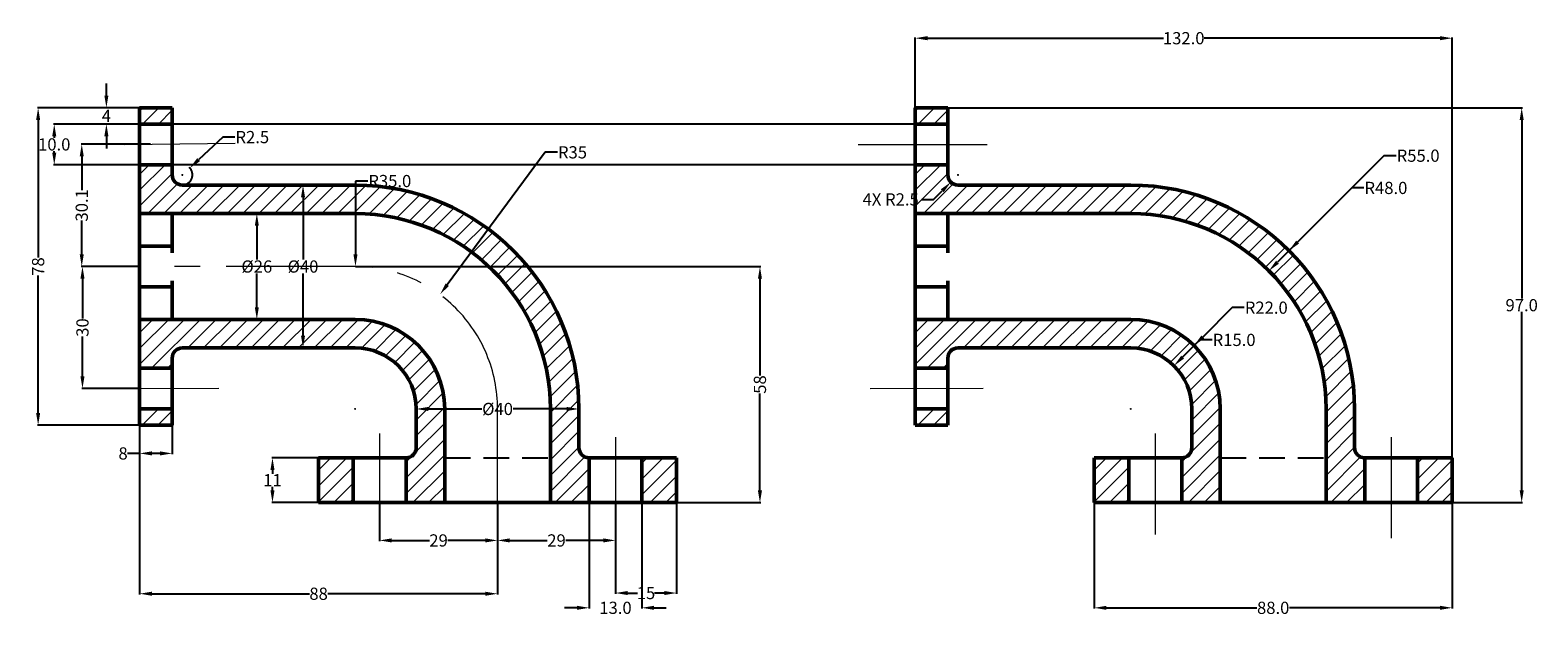
# Model space of a CAD drawing. Units: millimetres. Extents: x 96 to 467, y 38 to 182.
import ezdxf

# ---------------------------------------------------------------- set-up
doc = ezdxf.new("R2010")
doc.units = ezdxf.units.MM
doc.header["$MEASUREMENT"] = 0
doc.linetypes.add('CENTER', pattern=[50.8, 31.75, -6.35, 6.35, -6.35])
doc.linetypes.add('HIDDEN', pattern=[9.525, 6.35, -3.175])
for name, color, linetype, lineweight in [('M-CNTR', 1, 'CENTER', 18), ('M-DIMS', 3, 'Continuous', 25), ('M-HATC', 8, 'Continuous', 18), ('M-HIDN', 4, 'HIDDEN', 25), ('M-OUTL', 7, 'Continuous', 50)]:
    doc.layers.add(name, color=color, linetype=linetype, lineweight=lineweight)
doc.styles.get("Standard").update_dxf_attribs({"font": 'arial.ttf'})
doc.dimstyles.get("Standard").update_dxf_attribs({"dimtxt": 3, "dimasz": 3, "dimexe": 0.18, "dimexo": 0.0625, "dimgap": 0.09, "dimtad": 0, "dimtih": 1, "dimtoh": 1, "dimdec": 1, "dimdsep": 46, "dimtxsty": 'Standard', "dimcen": 0.09, "dimadec": 0, "dimazin": 0, "dimtfac": 1, "dimtdec": 1, "dimtofl": 0, "dimtmove": 0, "dimatfit": 3, "dimfxl": 1, "dimtolj": 1, "dimtzin": 0, "dimarcsym": 0})

# ---------------------------------------------------------------- blocks, each defined once
blk = doc.blocks.new('*D1')
at = {"layer": 'Defpoints', "color": 0, "transparency": 16777216}
for p in [(122.94, 84.65), (130.94, 84.65), (122.94, 77.73)]:
    blk.add_point(p, dxfattribs=at)
at = {"layer": 'M-DIMS', "color": 0, "lineweight": -2, "transparency": 16777216}
for p, q in [((122.94, 84.59), (122.94, 77.55)), ((130.94, 84.59), (130.94, 77.55)), ((122.94, 77.73), (119.94, 77.73)), ((127.94, 77.73), (125.94, 77.73))]:
    blk.add_line(p, q, dxfattribs=at)
at = {"layer": 'M-DIMS', "color": 0, "transparency": 16777216}
for points in [[(125.94, 78.23), (125.94, 77.23), (122.94, 77.73)], [(127.94, 78.23), (127.94, 77.23), (130.94, 77.73)]]:
    blk.add_solid(points, dxfattribs=at)
at = {"layer": 'M-DIMS', "color": 0, "transparency": 16777216, "insert": (118.86, 77.73), "char_height": 3, "attachment_point": 5}
blk.add_mtext('\\A1;8', dxfattribs=at)
blk = doc.blocks.new('*D2')
at = {"layer": 'Defpoints', "color": 0, "transparency": 16777216}
for p in [(108.88, 123.65), (122.94, 123.65), (122.94, 93.66)]:
    blk.add_point(p, dxfattribs=at)
at = {"layer": 'M-DIMS', "color": 0, "lineweight": -2, "transparency": 16777216}
for p, q in [((122.88, 123.65), (108.7, 123.65)), ((108.88, 120.65), (108.88, 110.89)), ((108.88, 96.66), (108.88, 106.42)), ((122.88, 93.66), (108.7, 93.66))]:
    blk.add_line(p, q, dxfattribs=at)
at = {"layer": 'M-DIMS', "color": 0, "transparency": 16777216}
for points in [[(108.38, 120.65), (109.38, 120.65), (108.88, 123.65)], [(108.38, 96.66), (109.38, 96.66), (108.88, 93.66)]]:
    blk.add_solid(points, dxfattribs=at)
at = {"layer": 'M-DIMS', "color": 0, "transparency": 16777216, "insert": (108.88, 108.66), "char_height": 3, "attachment_point": 5, "rotation": 90}
blk.add_mtext('\\A1;30', dxfattribs=at)
blk = doc.blocks.new('*D3')
at = {"layer": 'Defpoints', "color": 0, "transparency": 16777216}
for p in [(108.7, 153.71), (125.71, 153.71), (122.94, 123.65)]:
    blk.add_point(p, dxfattribs=at)
at = {"layer": 'M-DIMS', "color": 0, "lineweight": -2, "transparency": 16777216}
for p, q in [((125.64, 153.71), (108.52, 153.71)), ((108.7, 150.71), (108.7, 142.38)), ((108.7, 126.65), (108.7, 134.99)), ((122.88, 123.65), (108.52, 123.65))]:
    blk.add_line(p, q, dxfattribs=at)
at = {"layer": 'M-DIMS', "color": 0, "transparency": 16777216}
for points in [[(108.2, 150.71), (109.2, 150.71), (108.7, 153.71)], [(108.2, 126.65), (109.2, 126.65), (108.7, 123.65)]]:
    blk.add_solid(points, dxfattribs=at)
at = {"layer": 'M-DIMS', "color": 0, "transparency": 16777216, "insert": (108.7, 138.68), "char_height": 3, "attachment_point": 5, "rotation": 90}
blk.add_mtext('\\A1;30.1', dxfattribs=at)
blk = doc.blocks.new('*D4')
at = {"layer": 'Defpoints', "color": 0, "transparency": 16777216}
for p in [(122.94, 162.65), (114.76, 158.65), (122.94, 158.65)]:
    blk.add_point(p, dxfattribs=at)
at = {"layer": 'M-DIMS', "color": 0, "lineweight": -2, "transparency": 16777216}
for p, q in [((114.76, 165.65), (114.76, 168.65)), ((122.88, 162.65), (114.58, 162.65)), ((122.88, 158.65), (114.58, 158.65)), ((114.76, 155.65), (114.76, 152.65))]:
    blk.add_line(p, q, dxfattribs=at)
at = {"layer": 'M-DIMS', "color": 0, "transparency": 16777216}
for points in [[(114.26, 165.65), (115.26, 165.65), (114.76, 162.65)], [(114.26, 155.65), (115.26, 155.65), (114.76, 158.65)]]:
    blk.add_solid(points, dxfattribs=at)
at = {"layer": 'M-DIMS', "color": 0, "transparency": 16777216, "insert": (114.76, 160.65), "char_height": 3, "attachment_point": 5}
blk.add_mtext('\\A1;4', dxfattribs=at)
blk = doc.blocks.new('*D5')
at = {"layer": 'Defpoints', "color": 0, "transparency": 16777216}
for p in [(122.94, 162.65), (97.98, 84.65), (122.94, 84.65)]:
    blk.add_point(p, dxfattribs=at)
at = {"layer": 'M-DIMS', "color": 0, "lineweight": -2, "transparency": 16777216}
for p, q in [((122.88, 162.65), (97.8, 162.65)), ((97.98, 159.65), (97.98, 125.88)), ((97.98, 87.65), (97.98, 121.42)), ((122.88, 84.65), (97.8, 84.65))]:
    blk.add_line(p, q, dxfattribs=at)
at = {"layer": 'M-DIMS', "color": 0, "transparency": 16777216}
for points in [[(97.48, 159.65), (98.48, 159.65), (97.98, 162.65)], [(97.48, 87.65), (98.48, 87.65), (97.98, 84.65)]]:
    blk.add_solid(points, dxfattribs=at)
at = {"layer": 'M-DIMS', "color": 0, "transparency": 16777216, "insert": (97.98, 123.65), "char_height": 3, "attachment_point": 5, "rotation": 90}
blk.add_mtext('\\A1;78', dxfattribs=at)
blk = doc.blocks.new('*D6')
at = {"layer": 'Defpoints', "color": 0, "transparency": 16777216}
for p in [(133.44, 146.15), (135.27, 147.86)]:
    blk.add_point(p, dxfattribs=at)
at = {"layer": 'M-DIMS', "color": 0, "lineweight": -2, "transparency": 16777216}
for p, q in [((143.37, 155.45), (137.46, 149.91)), ((146.37, 155.45), (143.37, 155.45)), ((133.35, 146.15), (133.53, 146.15)), ((133.44, 146.06), (133.44, 146.24))]:
    blk.add_line(p, q, dxfattribs=at)
blk.add_arc((133.44, 146.15), 2.5, 271.4324, 47.2509, dxfattribs=at)
at = {"layer": 'M-DIMS', "color": 0, "transparency": 16777216}
blk.add_solid([(137.11, 150.28), (137.8, 149.55), (135.27, 147.86)], dxfattribs=at)
at = {"layer": 'M-DIMS', "color": 0, "transparency": 16777216, "insert": (150.64, 155.45), "char_height": 3, "attachment_point": 5}
blk.add_mtext('\\A1;R2.5', dxfattribs=at)
blk = doc.blocks.new('*D7')
at = {"layer": 'Defpoints', "color": 0, "transparency": 16777216}
for p in [(196.79, 116.77), (175.94, 88.65)]:
    blk.add_point(p, dxfattribs=at)
at = {"layer": 'M-DIMS', "color": 0, "lineweight": -2, "transparency": 16777216}
for p, q in [((222.69, 151.71), (198.57, 119.18)), ((225.69, 151.71), (222.69, 151.71)), ((175.85, 88.65), (176.03, 88.65)), ((175.94, 88.56), (175.94, 88.74))]:
    blk.add_line(p, q, dxfattribs=at)
at = {"layer": 'M-DIMS', "color": 0, "transparency": 16777216}
blk.add_solid([(198.17, 119.47), (198.97, 118.88), (196.79, 116.77)], dxfattribs=at)
at = {"layer": 'M-DIMS', "color": 0, "transparency": 16777216, "insert": (229.37, 151.71), "char_height": 3, "attachment_point": 5}
blk.add_mtext('\\A1;R35', dxfattribs=at)
blk = doc.blocks.new('*D8')
at = {"layer": 'Defpoints', "color": 0, "transparency": 16777216}
for p in [(149.44, 136.65), (149.44, 110.65), (151.75, 110.65)]:
    blk.add_point(p, dxfattribs=at)
at = {"layer": 'M-DIMS', "color": 0, "lineweight": -2, "transparency": 16777216}
for p, q in [((149.5, 136.65), (151.93, 136.65)), ((151.75, 133.65), (151.75, 125.36)), ((151.75, 113.65), (151.75, 121.95)), ((149.5, 110.65), (151.93, 110.65))]:
    blk.add_line(p, q, dxfattribs=at)
at = {"layer": 'M-DIMS', "color": 0, "transparency": 16777216}
for points in [[(151.25, 133.65), (152.25, 133.65), (151.75, 136.65)], [(151.25, 113.65), (152.25, 113.65), (151.75, 110.65)]]:
    blk.add_solid(points, dxfattribs=at)
at = {"layer": 'M-DIMS', "color": 0, "transparency": 16777216, "insert": (151.75, 123.65), "char_height": 3, "attachment_point": 5}
blk.add_mtext('\\A1;%%C26', dxfattribs=at)
blk = doc.blocks.new('*D9')
at = {"layer": 'Defpoints', "color": 0, "transparency": 16777216}
for p in [(154.69, 143.65), (154.69, 103.65), (163.11, 103.65)]:
    blk.add_point(p, dxfattribs=at)
at = {"layer": 'M-DIMS', "color": 0, "lineweight": -2, "transparency": 16777216}
for p, q in [((154.75, 143.65), (163.29, 143.65)), ((163.11, 140.65), (163.11, 125.36)), ((163.11, 106.65), (163.11, 121.95)), ((154.75, 103.65), (163.29, 103.65))]:
    blk.add_line(p, q, dxfattribs=at)
at = {"layer": 'M-DIMS', "color": 0, "transparency": 16777216}
for points in [[(162.61, 140.65), (163.61, 140.65), (163.11, 143.65)], [(162.61, 106.65), (163.61, 106.65), (163.11, 103.65)]]:
    blk.add_solid(points, dxfattribs=at)
at = {"layer": 'M-DIMS', "color": 0, "transparency": 16777216, "insert": (163.11, 123.65), "char_height": 3, "attachment_point": 5}
blk.add_mtext('\\A1;%%C40', dxfattribs=at)
blk = doc.blocks.new('*D10')
at = {"layer": 'Defpoints', "color": 0, "transparency": 16777216}
for p in [(190.94, 88.65), (230.94, 88.65), (230.94, 88.65)]:
    blk.add_point(p, dxfattribs=at)
at = {"layer": 'M-DIMS', "color": 0, "lineweight": -2, "transparency": 16777216}
for p, q in [((190.94, 88.71), (190.94, 88.83)), ((193.94, 88.65), (207.08, 88.65)), ((227.94, 88.65), (214.81, 88.65)), ((230.94, 88.71), (230.94, 88.83))]:
    blk.add_line(p, q, dxfattribs=at)
at = {"layer": 'M-DIMS', "color": 0, "transparency": 16777216}
for points in [[(193.94, 89.15), (193.94, 88.15), (190.94, 88.65)], [(227.94, 89.15), (227.94, 88.15), (230.94, 88.65)]]:
    blk.add_solid(points, dxfattribs=at)
at = {"layer": 'M-DIMS', "color": 0, "transparency": 16777216, "insert": (210.94, 88.65), "char_height": 3, "attachment_point": 5}
blk.add_mtext('\\A1;%%C40', dxfattribs=at)
blk = doc.blocks.new('*D11')
at = {"layer": 'Defpoints', "color": 0, "transparency": 16777216}
for p in [(155.6, 76.65), (166.94, 76.65), (166.94, 65.65)]:
    blk.add_point(p, dxfattribs=at)
at = {"layer": 'M-DIMS', "color": 0, "lineweight": -2, "transparency": 16777216}
for p, q in [((166.88, 76.65), (155.42, 76.65)), ((155.6, 73.65), (155.6, 72.75)), ((155.6, 68.65), (155.6, 69.55)), ((166.88, 65.65), (155.42, 65.65))]:
    blk.add_line(p, q, dxfattribs=at)
at = {"layer": 'M-DIMS', "color": 0, "transparency": 16777216}
for points in [[(155.1, 73.65), (156.1, 73.65), (155.6, 76.65)], [(155.1, 68.65), (156.1, 68.65), (155.6, 65.65)]]:
    blk.add_solid(points, dxfattribs=at)
at = {"layer": 'M-DIMS', "color": 0, "transparency": 16777216, "insert": (155.6, 71.15), "char_height": 3, "attachment_point": 5}
blk.add_mtext('\\A1;11', dxfattribs=at)
blk = doc.blocks.new('*D12')
at = {"layer": 'Defpoints', "color": 0, "transparency": 16777216}
for p in [(122.94, 84.65), (210.94, 65.65), (210.94, 43.25)]:
    blk.add_point(p, dxfattribs=at)
at = {"layer": 'M-DIMS', "color": 0, "lineweight": -2, "transparency": 16777216}
for p, q in [((122.94, 84.59), (122.94, 43.07)), ((210.94, 65.59), (210.94, 43.07)), ((125.94, 43.25), (164.7, 43.25)), ((207.94, 43.25), (169.18, 43.25))]:
    blk.add_line(p, q, dxfattribs=at)
at = {"layer": 'M-DIMS', "color": 0, "transparency": 16777216}
for points in [[(125.94, 43.75), (125.94, 42.75), (122.94, 43.25)], [(207.94, 43.75), (207.94, 42.75), (210.94, 43.25)]]:
    blk.add_solid(points, dxfattribs=at)
at = {"layer": 'M-DIMS', "color": 0, "transparency": 16777216, "insert": (166.94, 43.25), "char_height": 3, "attachment_point": 5}
blk.add_mtext('\\A1;88', dxfattribs=at)
blk = doc.blocks.new('*D13')
at = {"layer": 'Defpoints', "color": 0, "transparency": 16777216}
for p in [(181.94, 65.65), (210.94, 65.65), (181.94, 56.35)]:
    blk.add_point(p, dxfattribs=at)
at = {"layer": 'M-DIMS', "color": 0, "lineweight": -2, "transparency": 16777216}
for p, q in [((181.94, 65.59), (181.94, 56.17)), ((210.94, 65.59), (210.94, 56.17)), ((184.94, 56.35), (194.17, 56.35)), ((207.94, 56.35), (198.71, 56.35))]:
    blk.add_line(p, q, dxfattribs=at)
at = {"layer": 'M-DIMS', "color": 0, "transparency": 16777216}
for points in [[(184.94, 56.85), (184.94, 55.85), (181.94, 56.35)], [(207.94, 56.85), (207.94, 55.85), (210.94, 56.35)]]:
    blk.add_solid(points, dxfattribs=at)
at = {"layer": 'M-DIMS', "color": 0, "transparency": 16777216, "insert": (196.44, 56.35), "char_height": 3, "attachment_point": 5}
blk.add_mtext('\\A1;29', dxfattribs=at)
blk = doc.blocks.new('*D14')
at = {"layer": 'Defpoints', "color": 0, "transparency": 16777216}
for p in [(210.94, 65.65), (239.94, 65.65), (239.94, 56.35)]:
    blk.add_point(p, dxfattribs=at)
at = {"layer": 'M-DIMS', "color": 0, "lineweight": -2, "transparency": 16777216}
for p, q in [((210.94, 65.59), (210.94, 56.17)), ((239.94, 65.59), (239.94, 56.17)), ((213.94, 56.35), (223.17, 56.35)), ((236.94, 56.35), (227.71, 56.35))]:
    blk.add_line(p, q, dxfattribs=at)
at = {"layer": 'M-DIMS', "color": 0, "transparency": 16777216}
for points in [[(213.94, 56.85), (213.94, 55.85), (210.94, 56.35)], [(236.94, 56.85), (236.94, 55.85), (239.94, 56.35)]]:
    blk.add_solid(points, dxfattribs=at)
at = {"layer": 'M-DIMS', "color": 0, "transparency": 16777216, "insert": (225.44, 56.35), "char_height": 3, "attachment_point": 5}
blk.add_mtext('\\A1;29', dxfattribs=at)
blk = doc.blocks.new('*D15')
at = {"layer": 'Defpoints', "color": 0, "transparency": 16777216}
for p in [(239.94, 65.65), (254.94, 65.65), (254.94, 43.42)]:
    blk.add_point(p, dxfattribs=at)
at = {"layer": 'M-DIMS', "color": 0, "lineweight": -2, "transparency": 16777216}
for p, q in [((239.94, 65.59), (239.94, 43.24)), ((254.94, 65.59), (254.94, 43.24)), ((242.94, 43.42), (245.33, 43.42)), ((251.94, 43.42), (249.55, 43.42))]:
    blk.add_line(p, q, dxfattribs=at)
at = {"layer": 'M-DIMS', "color": 0, "transparency": 16777216}
for points in [[(242.94, 43.92), (242.94, 42.92), (239.94, 43.42)], [(251.94, 43.92), (251.94, 42.92), (254.94, 43.42)]]:
    blk.add_solid(points, dxfattribs=at)
at = {"layer": 'M-DIMS', "color": 0, "transparency": 16777216, "insert": (247.44, 43.42), "char_height": 3, "attachment_point": 5}
blk.add_mtext('\\A1;15', dxfattribs=at)
blk = doc.blocks.new('*D16')
at = {"layer": 'Defpoints', "color": 0, "transparency": 16777216}
for p in [(175.94, 123.65), (275.46, 123.65), (254.94, 65.65)]:
    blk.add_point(p, dxfattribs=at)
at = {"layer": 'M-DIMS', "color": 0, "lineweight": -2, "transparency": 16777216}
for p, q in [((176, 123.65), (275.64, 123.65)), ((275.46, 120.65), (275.46, 96.89)), ((275.46, 68.65), (275.46, 92.41)), ((255, 65.65), (275.64, 65.65))]:
    blk.add_line(p, q, dxfattribs=at)
at = {"layer": 'M-DIMS', "color": 0, "transparency": 16777216}
for points in [[(274.96, 120.65), (275.96, 120.65), (275.46, 123.65)], [(274.96, 68.65), (275.96, 68.65), (275.46, 65.65)]]:
    blk.add_solid(points, dxfattribs=at)
at = {"layer": 'M-DIMS', "color": 0, "transparency": 16777216, "insert": (275.46, 94.65), "char_height": 3, "attachment_point": 5, "rotation": 90}
blk.add_mtext('\\A1;58', dxfattribs=at)
blk = doc.blocks.new('ELBOW-90-FLANGED-SECTION')
for p, q in [((0, 97), (0, 19)), ((0, 97), (8, 97)), ((8, 97), (8, 80.5)), ((0, 93), (8, 93)), ((0, 83), (8, 83)), ((10.5, 78), (53, 78)), ((0, 71), (53, 71)), ((8, 71), (8, 61.33)), ((8, 63), (0, 63)), ((8, 53), (0, 53)), ((8, 54.45), (8, 45)), ((0, 45), (53, 45)), ((10.5, 38), (53, 38)), ((8, 35.5), (8, 19)), ((0, 33), (8, 33)), ((0, 23), (8, 23)), ((68, 23), (68, 13.5)), ((75, 23), (75, 11)), ((101, 23), (101, 11)), ((108, 23), (108, 13.5)), ((0, 19), (8, 19)), ((44, 11), (65.5, 11)), ((44, 11), (44, 0)), ((65.5, 11), (44, 11)), ((52.5, 11), (52.5, 0)), ((65.5, 11), (65.5, 0)), ((75, 11), (75, 0)), ((101, 11), (101, 0)), ((110.5, 11), (110.5, 0)), ((110.5, 11), (132, 11)), ((123.5, 11), (123.5, 0)), ((132, 11), (132, 0)), ((44, 0), (132, 0))]:
    blk.add_line(p, q)
for centre, radius, start, end in [((10.5, 80.5), 2.5, 180, 270), ((53, 23), 55, 0, 90), ((53, 23), 48, 0, 90), ((53, 23), 22, 0, 90), ((10.5, 35.5), 2.5, 90, 180), ((53, 23), 15, 0, 90), ((65.5, 13.5), 2.5, 270, 0), ((110.5, 13.5), 2.5, 180, 270)]:
    blk.add_arc(centre, radius, start, end)
blk = doc.blocks.new('*D18')
at = {"layer": 'Defpoints', "color": 0, "transparency": 16777216}
for p in [(445.66, 179.75), (313.66, 162.65), (445.66, 76.65)]:
    blk.add_point(p, dxfattribs=at)
at = {"layer": 'M-DIMS', "color": 0, "lineweight": -2, "transparency": 16777216}
for p, q in [((313.66, 162.71), (313.66, 179.93)), ((316.66, 179.75), (374.65, 179.75)), ((442.66, 179.75), (384.66, 179.75)), ((445.66, 76.71), (445.66, 179.93))]:
    blk.add_line(p, q, dxfattribs=at)
at = {"layer": 'M-DIMS', "color": 0, "transparency": 16777216}
for points in [[(316.66, 180.25), (316.66, 179.25), (313.66, 179.75)], [(442.66, 180.25), (442.66, 179.25), (445.66, 179.75)]]:
    blk.add_solid(points, dxfattribs=at)
at = {"layer": 'M-DIMS', "color": 0, "transparency": 16777216, "insert": (379.66, 179.75), "char_height": 3, "attachment_point": 5}
blk.add_mtext('\\A1;132.0', dxfattribs=at)
blk = doc.blocks.new('*D19')
at = {"layer": 'Defpoints', "color": 0, "transparency": 16777216}
for p in [(313.66, 162.65), (445.66, 65.65), (462.76, 65.65)]:
    blk.add_point(p, dxfattribs=at)
at = {"layer": 'M-DIMS', "color": 0, "lineweight": -2, "transparency": 16777216}
for p, q in [((313.72, 162.65), (462.94, 162.65)), ((462.76, 159.65), (462.76, 115.77)), ((462.76, 68.65), (462.76, 112.53)), ((445.72, 65.65), (462.94, 65.65))]:
    blk.add_line(p, q, dxfattribs=at)
at = {"layer": 'M-DIMS', "color": 0, "transparency": 16777216}
for points in [[(462.26, 159.65), (463.26, 159.65), (462.76, 162.65)], [(462.26, 68.65), (463.26, 68.65), (462.76, 65.65)]]:
    blk.add_solid(points, dxfattribs=at)
at = {"layer": 'M-DIMS', "color": 0, "transparency": 16777216, "insert": (462.76, 114.15), "char_height": 3, "attachment_point": 5}
blk.add_mtext('\\A1;97.0', dxfattribs=at)
blk = doc.blocks.new('*D20')
at = {"layer": 'Defpoints', "color": 0, "transparency": 16777216}
for p in [(357.66, 65.65), (445.66, 65.65), (445.66, 39.79)]:
    blk.add_point(p, dxfattribs=at)
at = {"layer": 'M-DIMS', "color": 0, "lineweight": -2, "transparency": 16777216}
for p, q in [((357.66, 65.59), (357.66, 39.61)), ((445.66, 65.59), (445.66, 39.61)), ((360.66, 39.79), (397.67, 39.79)), ((442.66, 39.79), (405.64, 39.79))]:
    blk.add_line(p, q, dxfattribs=at)
at = {"layer": 'M-DIMS', "color": 0, "transparency": 16777216}
for points in [[(360.66, 40.29), (360.66, 39.29), (357.66, 39.79)], [(442.66, 40.29), (442.66, 39.29), (445.66, 39.79)]]:
    blk.add_solid(points, dxfattribs=at)
at = {"layer": 'M-DIMS', "color": 0, "transparency": 16777216, "insert": (401.66, 39.79), "char_height": 3, "attachment_point": 5}
blk.add_mtext('\\A1;88.0', dxfattribs=at)
blk = doc.blocks.new('*D21')
at = {"layer": 'Defpoints', "color": 0, "transparency": 16777216}
for p in [(233.440976, 65.650906), (246.440976, 65.650906), (246.440976, 39.793084)]:
    blk.add_point(p, dxfattribs=at)
at = {"layer": 'M-DIMS', "color": 0, "lineweight": -2, "transparency": 16777216}
for p, q in [((233.440976, 65.588406), (233.440976, 39.613084)), ((246.440976, 65.588406), (246.440976, 39.613084)), ((230.440976, 39.793084), (227.440976, 39.793084)), ((249.440976, 39.793084), (252.440976, 39.793084))]:
    blk.add_line(p, q, dxfattribs=at)
at = {"layer": 'M-DIMS', "color": 0, "transparency": 16777216}
for points in [[(230.440976, 40.293084), (230.440976, 39.293084), (233.440976, 39.793084)], [(249.440976, 40.293084), (249.440976, 39.293084), (246.440976, 39.793084)]]:
    blk.add_solid(points, dxfattribs=at)
at = {"layer": 'M-DIMS', "color": 0, "transparency": 16777216, "insert": (239.940976, 39.793084), "char_height": 3, "attachment_point": 5}
blk.add_mtext('\\A1;13.0', dxfattribs=at)
blk = doc.blocks.new('*D22')
at = {"layer": 'Defpoints', "color": 0, "transparency": 16777216}
for p in [(101.94, 158.65), (313.66, 158.65), (313.66, 148.65)]:
    blk.add_point(p, dxfattribs=at)
at = {"layer": 'M-DIMS', "color": 0, "lineweight": -2, "transparency": 16777216}
for p, q in [((313.6, 158.65), (101.76, 158.65)), ((101.94, 155.65), (101.94, 155.27)), ((101.94, 151.65), (101.94, 152.03)), ((313.6, 148.65), (101.76, 148.65))]:
    blk.add_line(p, q, dxfattribs=at)
at = {"layer": 'M-DIMS', "color": 0, "transparency": 16777216}
for points in [[(101.44, 155.65), (102.44, 155.65), (101.94, 158.65)], [(101.44, 151.65), (102.44, 151.65), (101.94, 148.65)]]:
    blk.add_solid(points, dxfattribs=at)
at = {"layer": 'M-DIMS', "color": 0, "transparency": 16777216, "insert": (101.94, 153.65), "char_height": 3, "attachment_point": 5}
blk.add_mtext('\\A1;10.0', dxfattribs=at)
blk = doc.blocks.new('*D23')
at = {"layer": 'Defpoints', "color": 0, "transparency": 16777216}
for p in [(176, 123.65), (175.94, 88.65)]:
    blk.add_point(p, dxfattribs=at)
at = {"layer": 'M-DIMS', "color": 0, "lineweight": -2, "transparency": 16777216}
for p, q in [((176.04, 144.65), (176.01, 126.65)), ((179.04, 144.65), (176.04, 144.65)), ((175.85, 88.65), (176.03, 88.65)), ((175.94, 88.56), (175.94, 88.74))]:
    blk.add_line(p, q, dxfattribs=at)
at = {"layer": 'M-DIMS', "color": 0, "transparency": 16777216}
blk.add_solid([(175.51, 126.65), (176.51, 126.65), (176, 123.65)], dxfattribs=at)
at = {"layer": 'M-DIMS', "color": 0, "transparency": 16777216, "insert": (184.45, 144.65), "char_height": 3, "attachment_point": 5}
blk.add_mtext('\\A1;R35.0', dxfattribs=at)
blk = doc.blocks.new('*D24')
at = {"layer": 'Defpoints', "color": 0, "transparency": 16777216}
for p in [(405.55, 127.54), (366.66, 88.65)]:
    blk.add_point(p, dxfattribs=at)
at = {"layer": 'M-DIMS', "color": 0, "lineweight": -2, "transparency": 16777216}
for p, q in [((428.88, 150.88), (407.67, 129.66)), ((431.88, 150.88), (428.88, 150.88)), ((366.57, 88.65), (366.75, 88.65)), ((366.66, 88.56), (366.66, 88.74))]:
    blk.add_line(p, q, dxfattribs=at)
at = {"layer": 'M-DIMS', "color": 0, "transparency": 16777216}
blk.add_solid([(407.32, 130.02), (408.02, 129.31), (405.55, 127.54)], dxfattribs=at)
at = {"layer": 'M-DIMS', "color": 0, "transparency": 16777216, "insert": (437.3, 150.88), "char_height": 3, "attachment_point": 5}
blk.add_mtext('\\A1;R55.0', dxfattribs=at)
blk = doc.blocks.new('*D25')
at = {"layer": 'Defpoints', "color": 0, "transparency": 16777216}
for p in [(400.6, 122.59), (366.66, 88.65)]:
    blk.add_point(p, dxfattribs=at)
at = {"layer": 'M-DIMS', "color": 0, "lineweight": -2, "transparency": 16777216}
for p, q in [((420.96, 142.96), (402.72, 124.71)), ((423.96, 142.96), (420.96, 142.96)), ((366.57, 88.65), (366.75, 88.65)), ((366.66, 88.56), (366.66, 88.74))]:
    blk.add_line(p, q, dxfattribs=at)
at = {"layer": 'M-DIMS', "color": 0, "transparency": 16777216}
blk.add_solid([(402.37, 125.07), (403.07, 124.36), (400.6, 122.59)], dxfattribs=at)
at = {"layer": 'M-DIMS', "color": 0, "transparency": 16777216, "insert": (429.38, 142.96), "char_height": 3, "attachment_point": 5}
blk.add_mtext('\\A1;R48.0', dxfattribs=at)
blk = doc.blocks.new('*D26')
at = {"layer": 'Defpoints', "color": 0, "transparency": 16777216}
for p in [(382.21, 104.21), (366.66, 88.65)]:
    blk.add_point(p, dxfattribs=at)
at = {"layer": 'M-DIMS', "color": 0, "lineweight": -2, "transparency": 16777216}
for p, q in [((391.55, 113.54), (384.34, 106.33)), ((394.55, 113.54), (391.55, 113.54)), ((366.57, 88.65), (366.75, 88.65)), ((366.66, 88.56), (366.66, 88.74))]:
    blk.add_line(p, q, dxfattribs=at)
at = {"layer": 'M-DIMS', "color": 0, "transparency": 16777216}
blk.add_solid([(383.98, 106.68), (384.69, 105.98), (382.21, 104.21)], dxfattribs=at)
at = {"layer": 'M-DIMS', "color": 0, "transparency": 16777216, "insert": (399.96, 113.54), "char_height": 3, "attachment_point": 5}
blk.add_mtext('\\A1;R22.0', dxfattribs=at)
blk = doc.blocks.new('*D27')
at = {"layer": 'Defpoints', "color": 0, "transparency": 16777216}
for p in [(377.26, 99.26), (366.66, 88.65)]:
    blk.add_point(p, dxfattribs=at)
at = {"layer": 'M-DIMS', "color": 0, "lineweight": -2, "transparency": 16777216}
for p, q in [((383.63, 105.62), (379.39, 101.38)), ((386.63, 105.62), (383.63, 105.62)), ((366.57, 88.65), (366.75, 88.65)), ((366.66, 88.56), (366.66, 88.74))]:
    blk.add_line(p, q, dxfattribs=at)
at = {"layer": 'M-DIMS', "color": 0, "transparency": 16777216}
blk.add_solid([(379.03, 101.73), (379.74, 101.03), (377.26, 99.26)], dxfattribs=at)
at = {"layer": 'M-DIMS', "color": 0, "transparency": 16777216, "insert": (392.05, 105.62), "char_height": 3, "attachment_point": 5}
blk.add_mtext('\\A1;R15.0', dxfattribs=at)
blk = doc.blocks.new('*D28')
at = {"layer": 'Defpoints', "color": 0, "transparency": 16777216}
for p in [(324.16, 146.15), (322.39, 144.38)]:
    blk.add_point(p, dxfattribs=at)
at = {"layer": 'M-DIMS', "color": 0, "lineweight": -2, "transparency": 16777216}
for p, q in [((324.07, 146.15), (324.25, 146.15)), ((324.16, 146.06), (324.16, 146.24)), ((318.15, 140.14), (320.27, 142.26)), ((315.15, 140.14), (318.15, 140.14))]:
    blk.add_line(p, q, dxfattribs=at)
at = {"layer": 'M-DIMS', "color": 0, "transparency": 16777216}
blk.add_solid([(319.92, 142.61), (320.63, 141.91), (322.39, 144.38)], dxfattribs=at)
at = {"layer": 'M-DIMS', "color": 0, "transparency": 16777216, "insert": (307.6, 140.14), "char_height": 3, "attachment_point": 5}
blk.add_mtext('\\A1;4X R2.5', dxfattribs=at)

msp = doc.modelspace()

# ---------------------------------------------------------------- hatches: boundary and pattern name
at = {"layer": 'M-HATC'}
h = msp.add_hatch(dxfattribs=at)
h.set_pattern_fill('ANSI31', color=256, scale=22)
h.paths.add_polyline_path([(130.94, 88.65), (122.94, 88.65), (122.94, 84.65), (130.94, 84.65)], flags=16)
h.paths.add_polyline_path([(130.94, 162.65), (122.94, 162.65), (122.94, 158.65), (130.94, 158.65)])
h.paths.add_polyline_path([(175.94, 143.65), (133.44, 143.65, -0.414214), (130.94, 146.15), (130.94, 148.65), (122.94, 148.65), (122.94, 136.65), (175.94, 136.65, -0.414214), (223.94, 88.65), (223.94, 76.65), (223.94, 65.65), (233.44, 65.65), (233.44, 76.65, -0.414214), (230.94, 79.15), (230.94, 88.65, 0.414214)])
h.paths.add_polyline_path([(175.94, 110.65), (122.94, 110.65), (122.94, 98.65), (130.94, 98.65), (130.94, 101.15, -0.414214), (133.44, 103.65), (175.94, 103.65, -0.414214), (190.94, 88.65), (190.94, 79.15, -0.414214), (188.44, 76.65), (188.44, 65.65), (197.94, 65.65), (197.94, 76.65), (197.94, 88.65, 0.414214)], flags=17)
h.paths.add_polyline_path([(175.44, 76.65), (166.94, 76.65), (166.94, 65.65), (175.44, 65.65)], flags=16)
h.paths.add_polyline_path([(254.94, 76.65), (246.44, 76.65), (246.44, 65.65), (254.94, 65.65)])
h = msp.add_hatch(dxfattribs=at)
h.set_pattern_fill('ANSI31', color=256, scale=22)
h.set_pattern_definition([(45, (190.7172, 0), (-1.944544, 1.944544), [])])
h.paths.add_polyline_path([(321.66, 88.65), (313.66, 88.65), (313.66, 84.65), (321.66, 84.65)], flags=16)
h.paths.add_polyline_path([(321.66, 162.65), (313.66, 162.65), (313.66, 158.65), (321.66, 158.65)])
h.paths.add_polyline_path([(366.66, 143.65), (324.16, 143.65, -0.414214), (321.66, 146.15), (321.66, 148.65), (313.66, 148.65), (313.66, 136.65), (366.66, 136.65, -0.414214), (414.66, 88.65), (414.66, 76.65), (414.66, 65.65), (424.16, 65.65), (424.16, 76.65, -0.414214), (421.66, 79.15), (421.66, 88.65, 0.414214)])
h.paths.add_polyline_path([(366.66, 110.65), (313.66, 110.65), (313.66, 98.65), (321.66, 98.65), (321.66, 101.15, -0.414214), (324.16, 103.65), (366.66, 103.65, -0.414214), (381.66, 88.65), (381.66, 79.15, -0.414214), (379.16, 76.65), (379.16, 65.65), (388.66, 65.65), (388.66, 76.65), (388.66, 88.65, 0.414214)], flags=17)
h.paths.add_polyline_path([(366.16, 76.65), (357.66, 76.65), (357.66, 65.65), (366.16, 65.65)], flags=16)
h.paths.add_polyline_path([(445.66, 76.65), (437.16, 76.65), (437.16, 65.65), (445.66, 65.65)])

# ---------------------------------------------------------------- linework, layer by layer
at = {"layer": 'M-CNTR'}
for p, q in [((119.23, 153.65), (146.46, 153.92)), ((299.59, 153.65), (332.48, 153.65)), ((119.04, 93.65), (142.38, 93.72)), ((302.6, 93.65), (330.36, 93.72)), ((181.94, 82.64), (181.94, 57.77)), ((239.94, 81.73), (239.94, 56.89)), ((372.66, 82.64), (372.66, 57.77)), ((430.66, 81.73), (430.66, 56.89))]:
    msp.add_line(p, q, dxfattribs=at)
msp.add_lwpolyline([(210.94, 65.65), (210.94, 76.65), (210.94, 88.65, 0.414214), (175.94, 123.65), (130.94, 123.65)], format="xyb", dxfattribs=at)
at = {"layer": 'M-HIDN'}
for p, q in [((197.94, 76.65), (223.94, 76.65)), ((388.66, 76.65), (414.66, 76.65))]:
    msp.add_line(p, q, dxfattribs=at)

# ---------------------------------------------------------------- block references
at = {"layer": 'M-OUTL'}
for p in [(122.94, 65.65), (313.66, 65.65)]:
    msp.add_blockref('ELBOW-90-FLANGED-SECTION', p, dxfattribs=at)

# ---------------------------------------------------------------- dimensions: what is measured, and where the dimension line sits
at = {"layer": 'M-DIMS'}
for base, p1, p2, picture, middle in [((445.66, 179.75), (313.66, 162.65), (445.66, 76.65), '*D18', (379.66, 179.75)), ((246.44, 39.79), (233.44, 65.65), (246.44, 65.65), '*D21', (239.94, 39.79)), ((445.66, 39.79), (357.66, 65.65), (445.66, 65.65), '*D20', (401.66, 39.79))]:
    dim = msp.add_linear_dim(base=base, p1=p1, p2=p2, dimstyle='Standard', override={"dimdec": 1, "dimlfac": 1, "dimrnd": 0, "dimzin": 0, "dimdsep": 46, "dimlunit": 2}, dxfattribs=at)
    dim.commit()
    dim.dimension.update_dxf_attribs({"geometry": picture, "text_midpoint": middle})
at = {"layer": 'M-DIMS', "transparency": 33554610}
for base, p1, p2, picture, middle in [((114.76, 158.65), (122.94, 162.65), (122.94, 158.65), '*D4', (114.76, 160.65)), ((155.6, 76.65), (166.94, 65.65), (166.94, 76.65), '*D11', (155.6, 71.15))]:
    dim = msp.add_linear_dim(base=base, p1=p1, p2=p2, angle=90, dimstyle='Standard', override={"dimclrd": 0, "dimclre": 0, "dimclrt": 0}, dxfattribs=at)
    dim.commit()
    dim.dimension.update_dxf_attribs({"geometry": picture, "text_midpoint": middle})
for base, p1, p2, picture, middle in [((97.98, 84.65), (122.94, 162.65), (122.94, 84.65), '*D5', (97.98, 123.65)), ((108.7, 153.71), (122.94, 123.65), (125.71, 153.71), '*D3', (108.7, 138.68)), ((108.88, 123.65), (122.94, 93.66), (122.94, 123.65), '*D2', (108.88, 108.66)), ((275.46, 123.65), (254.94, 65.65), (175.94, 123.65), '*D16', (275.46, 94.65))]:
    dim = msp.add_linear_dim(base=base, p1=p1, p2=p2, angle=90, dimstyle='Standard', override={"dimclrd": 0, "dimclre": 0, "dimclrt": 0}, dxfattribs=at)
    dim.commit()
    dim.dimension.update_dxf_attribs({"geometry": picture, "text_midpoint": middle, "text_rotation": 90})
at = {"layer": 'M-DIMS'}
for base, p1, p2, picture, middle in [((462.76, 65.65), (313.66, 162.65), (445.66, 65.65), '*D19', (462.76, 114.15)), ((101.94, 158.65), (313.66, 148.65), (313.66, 158.65), '*D22', (101.94, 153.65))]:
    dim = msp.add_linear_dim(base=base, p1=p1, p2=p2, angle=90, dimstyle='Standard', override={"dimdec": 1, "dimlfac": 1, "dimrnd": 0, "dimzin": 0, "dimdsep": 46, "dimlunit": 2}, dxfattribs=at)
    dim.commit()
    dim.dimension.update_dxf_attribs({"geometry": picture, "text_midpoint": middle})
at = {"layer": 'M-DIMS', "transparency": 33554610}
for center, mpoint, picture, middle in [((133.44, 146.15), (135.27, 147.86), '*D6', (150.64, 155.45)), ((175.94, 88.65), (196.79, 116.77), '*D7', (229.37, 151.71))]:
    dim = msp.add_radius_dim(center=center, mpoint=mpoint, dimstyle='Standard', override={"dimclrd": 0, "dimclre": 0, "dimclrt": 0}, dxfattribs=at)
    dim.commit()
    dim.dimension.update_dxf_attribs({"geometry": picture, "text_midpoint": middle, "dimtype": 164})
at = {"layer": 'M-DIMS'}
for center, mpoint, picture, middle in [((366.66, 88.65), (405.55, 127.54), '*D24', (437.3, 150.88)), ((175.94, 88.65), (176, 123.65), '*D23', (184.45, 144.65)), ((366.66, 88.65), (400.6, 122.59), '*D25', (429.38, 142.96)), ((366.66, 88.65), (382.21, 104.21), '*D26', (399.96, 113.54)), ((366.66, 88.65), (377.26, 99.26), '*D27', (392.05, 105.62))]:
    dim = msp.add_radius_dim(center=center, mpoint=mpoint, dimstyle='Standard', override={"dimdec": 1, "dimlfac": 1, "dimrnd": 0, "dimzin": 0, "dimdsep": 46, "dimlunit": 2}, dxfattribs=at)
    dim.commit()
    dim.dimension.update_dxf_attribs({"geometry": picture, "text_midpoint": middle, "dimtype": 164})
dim = msp.add_radius_dim(center=(324.16, 146.15), mpoint=(322.39, 144.38), text='4X <>', dimstyle='Standard', override={"dimdec": 1, "dimlfac": 1, "dimrnd": 0, "dimzin": 0, "dimdsep": 46, "dimlunit": 2}, dxfattribs=at)
dim.commit()
dim.dimension.update_dxf_attribs({"geometry": '*D28', "text_midpoint": (307.6, 140.14)})
at = {"layer": 'M-DIMS', "transparency": 33554610}
for base, p1, p2, picture, middle in [((163.11, 103.65), (154.69, 143.65), (154.69, 103.65), '*D9', (163.11, 123.65)), ((151.75, 110.65), (149.44, 136.65), (149.44, 110.65), '*D8', (151.75, 123.65))]:
    dim = msp.add_linear_dim(base=base, p1=p1, p2=p2, angle=90, text='%%C<>', dimstyle='Standard', override={"dimclrd": 0, "dimclre": 0, "dimclrt": 0}, dxfattribs=at)
    dim.commit()
    dim.dimension.update_dxf_attribs({"geometry": picture, "text_midpoint": middle})
dim = msp.add_linear_dim(base=(230.94, 88.65), p1=(190.94, 88.65), p2=(230.94, 88.65), text='%%C<>', dimstyle='Standard', override={"dimclrd": 0, "dimclre": 0, "dimclrt": 0}, dxfattribs=at)
dim.commit()
dim.dimension.update_dxf_attribs({"geometry": '*D10', "text_midpoint": (210.94, 88.65)})
for base, p1, p2, picture, middle in [((122.94, 77.73), (130.94, 84.65), (122.94, 84.65), '*D1', (118.86, 77.73)), ((210.94, 43.25), (122.94, 84.65), (210.94, 65.65), '*D12', (166.94, 43.25)), ((181.94, 56.35), (210.94, 65.65), (181.94, 65.65), '*D13', (196.44, 56.35)), ((239.94, 56.35), (210.94, 65.65), (239.94, 65.65), '*D14', (225.44, 56.35)), ((254.94, 43.42), (239.94, 65.65), (254.94, 65.65), '*D15', (247.44, 43.42))]:
    dim = msp.add_linear_dim(base=base, p1=p1, p2=p2, dimstyle='Standard', override={"dimclrd": 0, "dimclre": 0, "dimclrt": 0}, dxfattribs=at)
    dim.commit()
    dim.dimension.update_dxf_attribs({"geometry": picture, "text_midpoint": middle})

doc.saveas('drawing.dxf')
